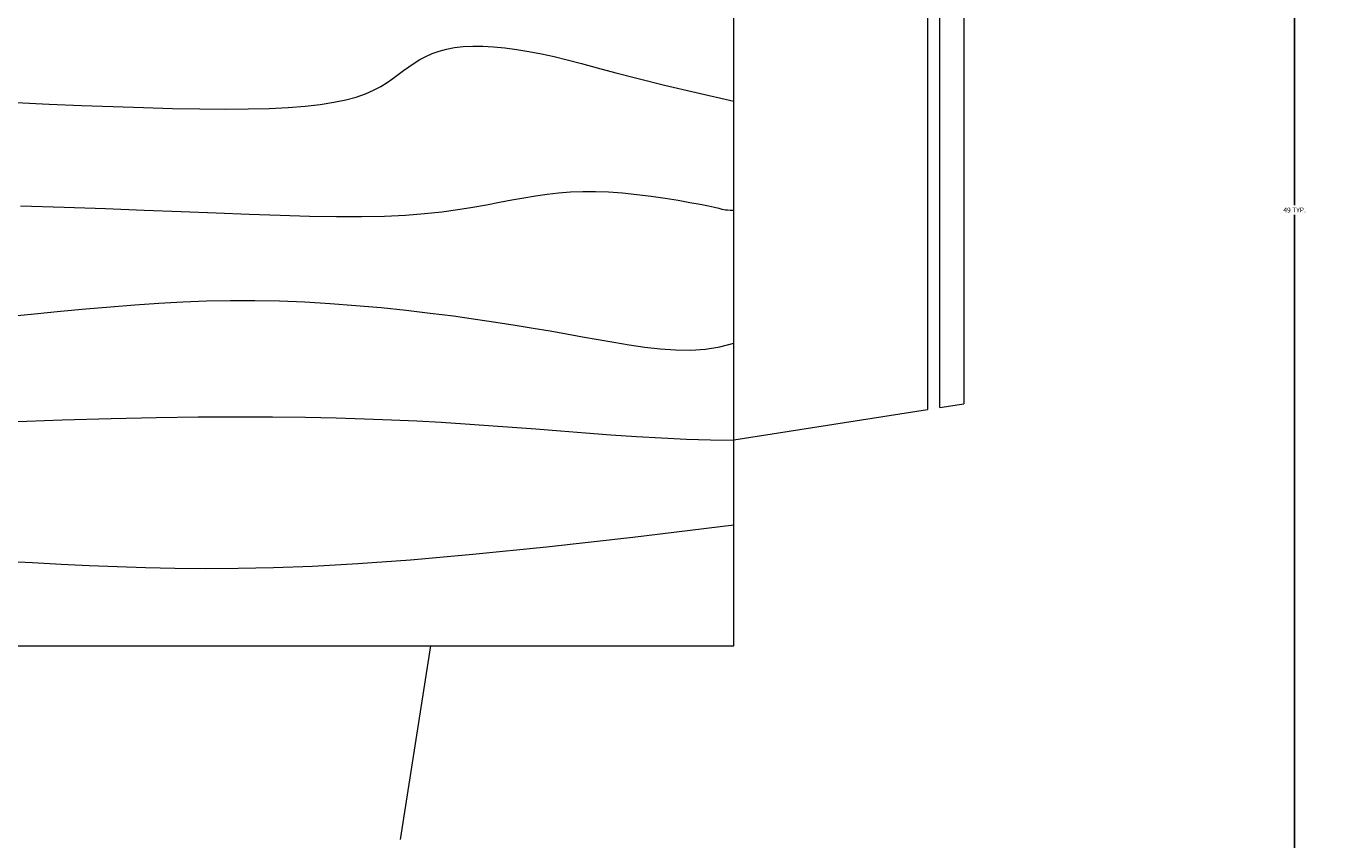
# Model space of a CAD drawing. Units: inches. Extents: x 4159 to 4826, y 299 to 1026.
# Tile 23 of 37: x 4354 to 4402, y 581 to 611. Entities that reach past the tile are written whole.
import ezdxf

# ---------------------------------------------------------------- set-up
doc = ezdxf.new("R2010")
doc.units = ezdxf.units.IN
doc.layers.add('A-ANNO-DIMS', color=2, linetype='Continuous', lineweight=18)
doc.layers.add('A-FURN', color=8, linetype='Continuous', lineweight=18)
doc.styles.get("Standard").update_dxf_attribs({"font": 'arial.ttf'})
doc.dimstyles.get("Standard").update_dxf_attribs({"dimtxt": 0.18, "dimasz": 0.18, "dimexe": 0.18, "dimexo": 0.0625, "dimgap": 0.09, "dimtad": 0, "dimtih": 1, "dimtoh": 1, "dimdec": 4, "dimzin": 0, "dimdsep": 46, "dimtxsty": 'Standard', "dimcen": 0.09, "dimadec": 0, "dimazin": 0, "dimtfac": 1, "dimtdec": 4, "dimtofl": 0, "dimtmove": 0, "dimatfit": 3, "dimfxl": 1, "dimtolj": 1, "dimtzin": 0, "dimarcsym": 0})

# ---------------------------------------------------------------- blocks, each defined once
blk = doc.blocks.new('Dining Set - 36 x 72 in.')
for p, q in [((36, -18), (36, 18)), ((44, 8.23041), (44, -8.23915)), ((44.5, -8.15843), (44.5, 8.15338)), ((45.5, 8), (45.5, -8)), ((44.4997, -8.15631), (45.5, -8)), ((35.9976, -9.48476), (43.9993, -8.2345)), ((-36, -18), (36, -18)), ((23.4848, -17.99762), (22.2345, -25.99928))]:
    blk.add_line(p, q)
for points in [[(6.373, 4.43782), (7.7344, 4.3776), (9.0723, 4.32129), (10.375, 4.27083), (11.6309, 4.22819), (12.8281, 4.19531), (13.9551, 4.17415), (15, 4.16666), (15.954, 4.17448), (16.819, 4.19791), (17.6001, 4.23698), (18.3021, 4.29166), (18.9299, 4.36198), (19.4883, 4.44791), (19.9823, 4.54948), (20.4167, 4.66666), (20.7969, 4.79899), (21.1302, 4.94401), (21.4245, 5.09879), (21.6875, 5.26041), (21.9271, 5.42594), (22.1511, 5.59245), (22.3672, 5.757), (22.5834, 5.91666), (22.8065, 6.06868), (23.0404, 6.21093), (23.2879, 6.34147), (23.5521, 6.45833), (23.8358, 6.55957), (24.142, 6.64323), (24.4735, 6.70735), (24.8334, 6.75), (25.2235, 6.76969), (25.642, 6.76692), (26.0858, 6.74267), (26.5521, 6.69791), (27.0379, 6.63362), (27.5404, 6.55078), (28.0565, 6.45036), (28.5834, 6.33333), (29.1242, 6.19987), (29.7071, 6.04687), (30.3661, 5.87044), (31.1354, 5.66666), (32.0493, 5.43164), (33.142, 5.16146), (34.4475, 4.85221), (36, 4.5)], [(6.5529, 0.17651), (8.3633, 0.12174), (10.0623, 0.06209), (11.6667, 0), (13.1899, -0.06201), (14.6341, -0.1211), (15.9982, -0.17432), (17.2813, -0.21875), (18.4823, -0.25147), (19.6003, -0.26953), (20.6343, -0.27002), (21.5834, -0.25), (22.4481, -0.20768), (23.2357, -0.14584), (23.9549, -0.06836), (24.6146, 0.02083), (25.2235, 0.11784), (25.7904, 0.21875), (26.3241, 0.31966), (26.8334, 0.41666), (27.3265, 0.50618), (27.8099, 0.58593), (28.2894, 0.65397), (28.7709, 0.70833), (29.2601, 0.74707), (29.763, 0.76823), (30.2855, 0.76985), (30.8334, 0.75), (31.4088, 0.70784), (31.9994, 0.64713), (32.589, 0.57275), (33.1615, 0.48958), (33.7008, 0.4025), (34.1908, 0.3164), (34.6153, 0.23616), (34.9584, 0.16666), (35.2099, 0.11165), (35.3848, 0.07031), (35.504, 0.04069), (35.5886, 0.02083), (35.6594, 0.00879), (35.7377, 0.0026), (35.8442, 0.00032), (36, 0)], [(6.0046, -4.39974), (7.127, -4.28646), (8.2053, -4.18099), (9.25, -4.08334), (10.2705, -3.99382), (11.2734, -3.91407), (12.2647, -3.84603), (13.25, -3.79167), (14.2354, -3.75293), (15.2266, -3.73177), (16.2295, -3.73015), (17.25, -3.75), (18.2912, -3.79248), (19.3451, -3.85547), (20.4009, -3.93604), (21.4479, -4.03125), (22.4754, -4.13819), (23.4727, -4.25391), (24.4289, -4.37549), (25.3334, -4.5), (26.1785, -4.62492), (26.9694, -4.74935), (27.7145, -4.87281), (28.4219, -4.99479), (29.1, -5.11483), (29.7572, -5.23242), (30.4016, -5.34709), (31.0417, -5.45834), (31.6837, -5.56437), (32.3262, -5.65821), (32.9658, -5.73153), (33.599, -5.77604), (34.2224, -5.78345), (34.8327, -5.74545), (35.4264, -5.65373), (36, -5.5)], [(6.0833, -8.75), (8.2767, -8.66765), (10.3021, -8.60677), (12.1712, -8.56543), (13.8958, -8.54167), (15.4876, -8.53353), (16.9583, -8.53907), (18.3197, -8.55632), (19.5834, -8.58334), (20.7616, -8.61841), (21.8685, -8.66081), (22.9188, -8.71004), (23.9271, -8.76563), (24.9081, -8.82707), (25.8763, -8.89388), (26.8465, -8.96558), (27.8334, -9.04167), (28.8474, -9.12118), (29.8828, -9.20117), (30.93, -9.27824), (31.9792, -9.34896), (33.0205, -9.40991), (34.0443, -9.45768), (35.0407, -9.48885), (36, -9.5)], [(5.8333, -14.5), (7.0554, -14.5621), (8.235, -14.62175), (9.3922, -14.67652), (10.5469, -14.72396), (11.7192, -14.76164), (12.929, -14.78711), (14.1965, -14.79794), (15.5417, -14.79167), (16.9933, -14.76424), (18.6152, -14.70508), (20.4804, -14.60197), (22.6615, -14.44271), (25.2312, -14.21509), (28.2624, -13.9069), (31.8277, -13.50594), (36, -13)]]:
    blk.add_lwpolyline(points)
blk = doc.blocks.new('*D36')
at = {"layer": 'A-ANNO-DIMS', "color": 0, "lineweight": -2, "transparency": 16777216}
for p, q in [((4388.337, 628.759), (4400.621, 628.759)), ((4400.441, 628.579), (4400.441, 604.428)), ((4400.441, 579.914), (4400.441, 604.064)), ((4388.337, 579.734), (4400.621, 579.734))]:
    blk.add_line(p, q, dxfattribs=at)
at = {"layer": 'A-ANNO-DIMS', "color": 0, "transparency": 16777216}
for points in [[(4400.411, 628.579), (4400.471, 628.579), (4400.441, 628.759)], [(4400.411, 579.914), (4400.471, 579.914), (4400.441, 579.734)]]:
    blk.add_solid(points, dxfattribs=at)
at = {"layer": 'Defpoints', "color": 0, "transparency": 16777216}
for p in [(4388.274, 628.759), (4400.441, 628.759), (4388.274, 579.734)]:
    blk.add_point(p, dxfattribs=at)
at = {"layer": 'A-ANNO-DIMS', "color": 0, "transparency": 16777216, "insert": (4400.441, 604.246), "char_height": 0.18, "attachment_point": 5}
blk.add_mtext('\\A1;49 TYP.', dxfattribs=at)
blk = doc.blocks.new('*D44')
at = {"layer": 'A-ANNO-DIMS', "color": 0, "lineweight": -2, "transparency": 16777216}
for p, q in [((4287.263, 963.093), (4158.88, 963.093)), ((4159.06, 962.913), (4159.06, 647.826)), ((4159.06, 332.375), (4159.06, 647.462)), ((4447.248, 332.195), (4158.88, 332.195))]:
    blk.add_line(p, q, dxfattribs=at)
at = {"layer": 'A-ANNO-DIMS', "color": 0, "transparency": 16777216}
for points in [[(4159.03, 962.913), (4159.09, 962.913), (4159.06, 963.093)], [(4159.03, 332.375), (4159.09, 332.375), (4159.06, 332.195)]]:
    blk.add_solid(points, dxfattribs=at)
at = {"layer": 'Defpoints', "color": 0, "transparency": 16777216}
for p in [(4287.326, 963.093), (4159.06, 332.195), (4447.31, 332.195)]:
    blk.add_point(p, dxfattribs=at)
at = {"layer": 'A-ANNO-DIMS', "color": 0, "transparency": 16777216, "insert": (4159.06, 647.644), "char_height": 0.18, "attachment_point": 5}
blk.add_mtext('\\A1;630.9', dxfattribs=at)

msp = doc.modelspace()

# ---------------------------------------------------------------- block references
at = {"layer": 'A-FURN', "xscale": 0.8913588978043845, "yscale": 0.8913588978043845, "zscale": 0.8913588978043845}
msp.add_blockref('Dining Set - 36 x 72 in.', (4347.717, 604.246), dxfattribs=at)

# ---------------------------------------------------------------- dimensions: what is measured, and where the dimension line sits
at = {"layer": 'A-ANNO-DIMS'}
dim = msp.add_linear_dim(base=(4159.06, 332.195), p1=(4287.326, 963.093), p2=(4447.31, 332.195), angle=90, dimstyle='Standard', override={"dimdec": 1, "dimlfac": 1, "dimrnd": 0, "dimzin": 0, "dimdsep": 46, "dimlunit": 2}, dxfattribs=at)
dim.commit()
dim.dimension.update_dxf_attribs({"geometry": '*D44', "text_midpoint": (4159.06, 647.644)})
dim = msp.add_linear_dim(base=(4400.441, 628.759), p1=(4388.274, 579.734), p2=(4388.274, 628.759), angle=90, text='<> TYP.', dimstyle='Standard', override={"dimdec": 0, "dimlfac": 1, "dimrnd": 0, "dimzin": 0, "dimdsep": 46, "dimlunit": 2}, dxfattribs=at)
dim.commit()
dim.dimension.update_dxf_attribs({"geometry": '*D36', "text_midpoint": (4400.441, 604.246)})

doc.saveas('drawing.dxf')
